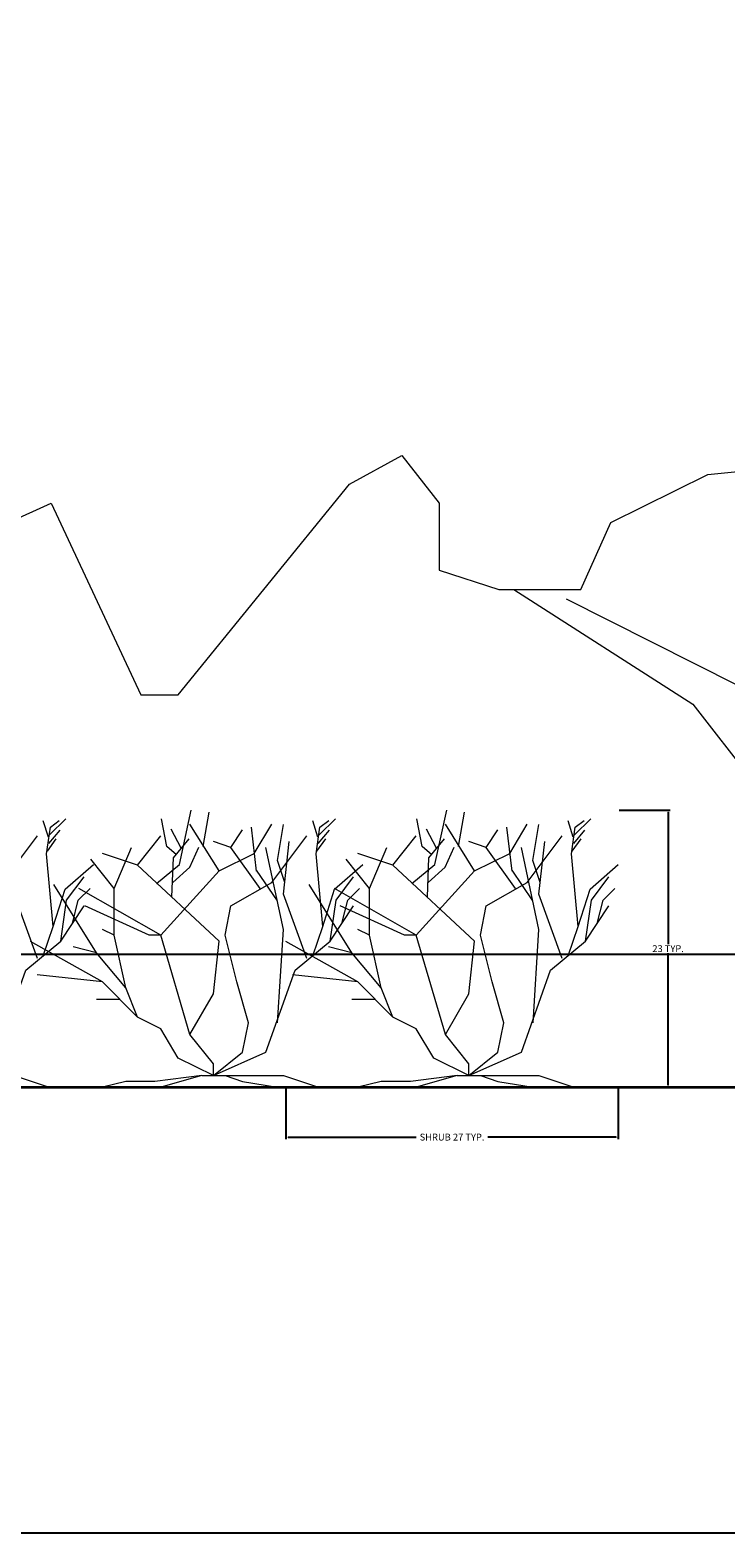
# Model space of a CAD drawing. Units: inches. Extents: x -26 to 776, y -22 to 650.
# Tile 45 of 62: x 584 to 642, y -22 to 102. Entities that reach past the tile are written whole.
import ezdxf

# ---------------------------------------------------------------- set-up
doc = ezdxf.new("R2010")
doc.units = ezdxf.units.IN
doc.header["$MEASUREMENT"] = 0
for name, color, linetype, lineweight in [('A-ANNO-DIMS', 2, 'Continuous', 18), ('C-TOPO', 7, 'Continuous', 35), ('L-PLNT-SHRB', 94, 'Continuous', 13), ('L-PLNT-TREE', 94, 'Continuous', 18)]:
    doc.layers.add(name, color=color, linetype=linetype, lineweight=lineweight)
doc.styles.get("Standard").update_dxf_attribs({"font": 'arial.ttf'})
doc.dimstyles.get("Standard").update_dxf_attribs({"dimtxt": 0.5625, "dimasz": 0.18, "dimexe": 0.18, "dimexo": 0.0625, "dimgap": 0.09, "dimtad": 0, "dimtih": 1, "dimtoh": 1, "dimdec": 4, "dimzin": 0, "dimdsep": 46, "dimlunit": 4, "dimtxsty": 'Standard', "dimcen": 0.09, "dimadec": 0, "dimazin": 0, "dimtfac": 1, "dimtdec": 4, "dimtofl": 0, "dimtmove": 0, "dimatfit": 3, "dimfxl": 1, "dimtolj": 1, "dimtzin": 0, "dimarcsym": 0})

# ---------------------------------------------------------------- blocks, each defined once
blk = doc.blocks.new('Tree - type 3 evergreen elevation')
for points in [[(-41.4085, 64.6985), (-44.3346, 59.8898), (-42.2089, 60.1377), (-42.5159, 55.7849), (-49.6039, 46.4502), (-58.2307, 45.8972), (-62.1127, 43.6853), (-68.5828, 36.4966), (-65.9947, 32.0727), (-50.0352, 32.6257), (-47.0159, 30.4138), (-39.6831, 33.7317), (-34.507, 22.6721), (-32.3504, 22.6721), (-22.4296, 34.8376), (-19.4102, 36.4966), (-17.2536, 33.7317), (-17.2536, 29.8608), (-13.8028, 28.7549), (-9.0581, 28.7549), (-7.3328, 32.6257), (-1.7254, 35.3906), (3.8821, 35.9436)], [(-9.9208, 28.2019), (0, 23.2251), (3.4507, 19.9072), (4.7447, 15.4834), (8.6267, 27.0959), (6.4701, 37.6025)], [(-12.9401, 28.7549), (-2.588, 22.1191), (0.8626, 17.6953), (1.7253, 11.6125), (0, 0)]]:
    blk.add_lwpolyline(points)
blk = doc.blocks.new('Shrub - elevation')
for p, q in [((-11.433, 18.289), (-10.457, 22.749)), ((-9.48, 19.775), (-8.992, 22.592)), ((-12.471, 19.775), (-12.898, 22.044)), ((-11.28, 19.619), (-12.104, 21.184)), ((-8.16, 17.76), (-10.56, 21.6)), ((-7.2, 19.68), (-6.24, 21.12)), ((-5.086, 17.741), (-5.513, 21.34)), ((-5.28, 19.2), (-3.84, 21.6)), ((-3.377, 18.602), (-2.888, 21.575)), ((-0.508, 21.888), (-0.081, 20.558)), ((-0.203, 19.149), (0.102, 21.34)), ((-0.02, 20.01), (0.896, 21.105)), ((0.041, 20.714), (1.384, 22.044)), ((0.102, 21.34), (0.835, 21.888)), ((-14.88, 18.24), (-12.96, 20.64)), ((-11.921, 18.836), (-10.64, 20.401)), ((-7.2, 19.68), (-8.64, 20.16)), ((-3.84, 16.8), (-0.96, 20.64)), ((-2.88, 15.84), (-2.4, 20.16)), ((-0.142, 19.384), (0.59, 20.401)), ((-16.8, 16.32), (-18.72, 18.72)), ((-14.88, 18.24), (-17.76, 19.2)), ((-16.8, 16.32), (-15.36, 19.68)), ((-11.677, 19.071), (-12.471, 19.775)), ((-12.043, 15.628), (-11.921, 18.836)), ((-10.579, 18.054), (-9.846, 19.697)), ((-8.16, 17.76), (-5.28, 19.2)), ((-4.8, 16.32), (-7.2, 19.68)), ((-2.88, 12.96), (-4.32, 19.68)), ((-2.766, 16.802), (-3.377, 18.602)), ((0.346, 13.203), (-0.203, 19.149)), ((-8.16, 12), (-14.88, 18.24)), ((-13.325, 16.724), (-11.433, 18.289)), ((-12.96, 12.48), (-8.16, 17.76)), ((-11.982, 16.802), (-10.579, 18.054)), ((-3.377, 15.315), (-5.086, 17.819)), ((1.323, 16.254), (3.642, 18.289)), ((-18.24, 11.04), (-21.755, 16.655)), ((-12.96, 12.48), (-19.68, 16.32)), ((-16.8, 12.48), (-16.8, 16.32)), ((-7.2, 14.88), (-3.84, 16.8)), ((0.346, 13.203), (1.323, 16.254)), ((1.44, 15.36), (2.88, 17.28)), ((2.4, 15.36), (3.36, 16.32)), ((-13.92, 12.48), (-19.2, 14.88)), ((-7.68, 12.48), (-7.2, 14.88)), ((-0.96, 10.56), (-2.88, 15.84)), ((0.96, 12), (1.44, 15.36)), ((0.96, 12), (2.88, 14.88)), ((1.92, 13.44), (2.4, 15.36)), ((-16.8, 12.48), (-17.76, 12.96)), ((-15.84, 8.16), (-16.8, 12.48)), ((-12.96, 12.48), (-13.92, 12.48)), ((-10.56, 4.32), (-12.96, 12.48)), ((-6.72, 8.64), (-7.68, 12.48)), ((-3.36, 5.28), (-2.88, 12.96)), ((-0.48, 10.8), (0.346, 13.203)), ((-17.76, 8.64), (-23.663, 11.961)), ((-18.24, 11.04), (-20.16, 11.52)), ((-8.64, 7.68), (-8.16, 12)), ((-1.92, 9.6), (0.96, 12)), ((-15.84, 8.16), (-18.24, 11.04)), ((-17.76, 8.64), (-23.128, 9.222)), ((-4.32, 2.88), (-1.92, 9.6)), ((-14.88, 5.76), (-17.76, 8.64)), ((-14.88, 5.76), (-15.84, 8.16)), ((-10.56, 4.32), (-8.64, 7.68)), ((-5.76, 5.28), (-6.72, 8.64)), ((-16.32, 7.2), (-18.24, 7.2)), ((-12.96, 4.8), (-14.88, 5.76)), ((-6.24, 2.88), (-5.76, 5.28)), ((-11.52, 2.4), (-12.96, 4.8)), ((-8.64, 1.92), (-10.56, 4.32)), ((-8.64, 0.96), (-4.32, 2.88)), ((-8.64, 0.96), (-6.24, 2.88)), ((-8.64, 0.96), (-11.52, 2.4)), ((-8.64, 0.96), (-8.64, 1.92)), ((-15.84, 0.48), (-17.76, 0)), ((-13.44, 0.48), (-15.84, 0.48)), ((-9.6, 0.96), (-13.44, 0.48)), ((-9.6, 0.96), (-12.96, 0)), ((-9.6, 0.96), (-7.68, 0.96)), ((-8.64, 0.96), (-2.88, 0.96)), ((-7.68, 0.96), (-6.24, 0.48)), ((-6.24, 0.48), (-3.36, 0)), ((-2.88, 0.96), (0, 0))]:
    blk.add_line(p, q)
blk = doc.blocks.new('*D11')
at = {"layer": 'A-ANNO-DIMS', "color": 0, "lineweight": -2, "transparency": 16777216}
for p, q in [((605.39, 15.42), (605.39, 11.21)), ((632.7, 15.42), (632.7, 11.21)), ((605.57, 11.39), (616.1, 11.39)), ((632.52, 11.39), (621.99, 11.39))]:
    blk.add_line(p, q, dxfattribs=at)
at = {"layer": 'A-ANNO-DIMS', "color": 0, "transparency": 16777216}
for points in [[(605.57, 11.42), (605.57, 11.36), (605.39, 11.39)], [(632.52, 11.42), (632.52, 11.36), (632.7, 11.39)]]:
    blk.add_solid(points, dxfattribs=at)
at = {"layer": 'Defpoints', "color": 0, "transparency": 16777216}
for p in [(605.39, 15.48), (632.7, 15.48), (632.7, 11.39)]:
    blk.add_point(p, dxfattribs=at)
at = {"layer": 'A-ANNO-DIMS', "color": 0, "transparency": 16777216, "insert": (619.04, 11.39), "char_height": 0.5625, "attachment_point": 5}
blk.add_mtext('\\A1;SHRUB 27 TYP.', dxfattribs=at)
blk = doc.blocks.new('*D12')
at = {"layer": 'A-ANNO-DIMS', "color": 0, "lineweight": -2, "transparency": 16777216}
for p, q in [((632.76, 38.23), (636.97, 38.23)), ((636.79, 38.05), (636.79, 27.23)), ((636.79, 15.66), (636.79, 26.48)), ((632.76, 15.48), (636.97, 15.48))]:
    blk.add_line(p, q, dxfattribs=at)
at = {"layer": 'A-ANNO-DIMS', "color": 0, "transparency": 16777216}
for points in [[(636.76, 38.05), (636.82, 38.05), (636.79, 38.23)], [(636.76, 15.66), (636.82, 15.66), (636.79, 15.48)]]:
    blk.add_solid(points, dxfattribs=at)
at = {"layer": 'Defpoints', "color": 0, "transparency": 16777216}
for p in [(632.7, 38.23), (636.79, 38.23), (632.7, 15.48)]:
    blk.add_point(p, dxfattribs=at)
at = {"layer": 'A-ANNO-DIMS', "color": 0, "transparency": 16777216, "insert": (636.79, 26.86), "char_height": 0.5625, "attachment_point": 5}
blk.add_mtext('\\A1;23 TYP.', dxfattribs=at)
blk = doc.blocks.new('*D13')
at = {"layer": 'A-ANNO-DIMS', "color": 0, "lineweight": -2, "transparency": 16777216}
for p, q in [((738.75, 50.79), (738.75, -21.31)), ((11.11, 15.42), (11.11, -21.31)), ((11.29, -21.13), (373.89, -21.13)), ((738.57, -21.13), (375.97, -21.13))]:
    blk.add_line(p, q, dxfattribs=at)
at = {"layer": 'A-ANNO-DIMS', "color": 0, "transparency": 16777216}
for points in [[(11.29, -21.1), (11.29, -21.16), (11.11, -21.13)], [(738.57, -21.1), (738.57, -21.16), (738.75, -21.13)]]:
    blk.add_solid(points, dxfattribs=at)
at = {"layer": 'Defpoints', "color": 0, "transparency": 16777216}
for p in [(738.75, 50.85), (11.11, 15.48), (738.75, -21.13)]:
    blk.add_point(p, dxfattribs=at)
at = {"layer": 'A-ANNO-DIMS', "color": 0, "transparency": 16777216, "insert": (374.93, -21.13), "char_height": 0.562, "attachment_point": 5}
blk.add_mtext('\\A1;727.6', dxfattribs=at)
blk = doc.blocks.new('*D20')
at = {"layer": 'A-ANNO-DIMS', "color": 0, "lineweight": -2, "transparency": 16777216}
for p, q in [((425.81, 455.47), (775.34, 455.47)), ((775.16, 455.29), (775.16, 235.85)), ((775.16, 15.66), (775.16, 235.1)), ((425.81, 15.48), (775.34, 15.48))]:
    blk.add_line(p, q, dxfattribs=at)
at = {"layer": 'A-ANNO-DIMS', "color": 0, "transparency": 16777216}
for points in [[(775.13, 455.29), (775.19, 455.29), (775.16, 455.47)], [(775.13, 15.66), (775.19, 15.66), (775.16, 15.48)]]:
    blk.add_solid(points, dxfattribs=at)
at = {"layer": 'Defpoints', "color": 0, "transparency": 16777216}
for p in [(425.74, 455.47), (775.16, 455.47), (425.74, 15.48)]:
    blk.add_point(p, dxfattribs=at)
at = {"layer": 'A-ANNO-DIMS', "color": 0, "transparency": 16777216, "insert": (775.16, 235.48), "char_height": 0.562, "attachment_point": 5}
blk.add_mtext('\\A1;440', dxfattribs=at)
blk = doc.blocks.new('*D30')
at = {"layer": 'A-ANNO-DIMS', "color": 0, "lineweight": -2, "transparency": 16777216}
for p, q in [((280.68, 144.84), (775.34, 144.84)), ((775.16, 144.66), (775.16, 86.01)), ((775.16, 26.6), (775.16, 85.25)), ((280.68, 26.42), (775.34, 26.42))]:
    blk.add_line(p, q, dxfattribs=at)
at = {"layer": 'A-ANNO-DIMS', "color": 0, "transparency": 16777216}
for points in [[(775.13, 144.66), (775.19, 144.66), (775.16, 144.84)], [(775.13, 26.6), (775.19, 26.6), (775.16, 26.42)]]:
    blk.add_solid(points, dxfattribs=at)
at = {"layer": 'Defpoints', "color": 0, "transparency": 16777216}
for p in [(280.62, 144.84), (775.16, 144.84), (280.62, 26.42)]:
    blk.add_point(p, dxfattribs=at)
at = {"layer": 'A-ANNO-DIMS', "color": 0, "transparency": 16777216, "insert": (775.16, 85.63), "char_height": 0.562, "attachment_point": 5}
blk.add_mtext('\\A1;118.41', dxfattribs=at)
blk = doc.blocks.new('*D38')
at = {"layer": 'A-ANNO-DIMS', "color": 0, "lineweight": -2, "transparency": 16777216}
for p, q in [((280.68, 26.42), (775.34, 26.42)), ((775.16, 26.24), (775.16, 21.33)), ((775.16, 15.66), (775.16, 20.58)), ((289.3, 15.48), (775.34, 15.48))]:
    blk.add_line(p, q, dxfattribs=at)
at = {"layer": 'A-ANNO-DIMS', "color": 0, "transparency": 16777216}
for points in [[(775.13, 26.24), (775.19, 26.24), (775.16, 26.42)], [(775.13, 15.66), (775.19, 15.66), (775.16, 15.48)]]:
    blk.add_solid(points, dxfattribs=at)
at = {"layer": 'Defpoints', "color": 0, "transparency": 16777216}
for p in [(280.62, 26.42), (775.16, 26.42), (289.24, 15.48)]:
    blk.add_point(p, dxfattribs=at)
at = {"layer": 'A-ANNO-DIMS', "color": 0, "transparency": 16777216, "insert": (775.16, 20.95), "char_height": 0.562, "attachment_point": 5}
blk.add_mtext('\\A1;10.942', dxfattribs=at)
blk = doc.blocks.new('*D45')
at = {"layer": 'A-ANNO-DIMS', "color": 0, "lineweight": -2, "transparency": 16777216}
for p, q in [((507.74, 408.64), (775.34, 408.64)), ((775.16, 408.46), (775.16, 212.44)), ((775.16, 15.66), (775.16, 211.68)), ((586, 15.48), (775.34, 15.48))]:
    blk.add_line(p, q, dxfattribs=at)
at = {"layer": 'A-ANNO-DIMS', "color": 0, "transparency": 16777216}
for points in [[(775.13, 408.46), (775.19, 408.46), (775.16, 408.64)], [(775.13, 15.66), (775.19, 15.66), (775.16, 15.48)]]:
    blk.add_solid(points, dxfattribs=at)
at = {"layer": 'Defpoints', "color": 0, "transparency": 16777216}
for p in [(507.68, 408.64), (775.16, 408.64), (585.94, 15.48)]:
    blk.add_point(p, dxfattribs=at)
at = {"layer": 'A-ANNO-DIMS', "color": 0, "transparency": 16777216, "insert": (775.16, 212.06), "char_height": 0.562, "attachment_point": 5}
blk.add_mtext('\\A1;393.16', dxfattribs=at)
blk = doc.blocks.new('*D48')
at = {"layer": 'A-ANNO-DIMS', "color": 0, "lineweight": -2, "transparency": 16777216}
for p, q in [((545.03, 67.41), (545.03, 649.86)), ((738.75, 50.91), (738.75, 649.86)), ((545.21, 649.68), (640.88, 649.68)), ((738.57, 649.68), (642.9, 649.68))]:
    blk.add_line(p, q, dxfattribs=at)
at = {"layer": 'A-ANNO-DIMS', "color": 0, "transparency": 16777216}
for points in [[(545.21, 649.71), (545.21, 649.65), (545.03, 649.68)], [(738.57, 649.71), (738.57, 649.65), (738.75, 649.68)]]:
    blk.add_solid(points, dxfattribs=at)
at = {"layer": 'Defpoints', "color": 0, "transparency": 16777216}
for p in [(738.75, 649.68), (545.03, 67.35), (738.75, 50.85)]:
    blk.add_point(p, dxfattribs=at)
at = {"layer": 'A-ANNO-DIMS', "color": 0, "transparency": 16777216, "insert": (641.89, 649.68), "char_height": 0.562, "attachment_point": 5}
blk.add_mtext('\\A1;193.7', dxfattribs=at)

msp = doc.modelspace()

# ---------------------------------------------------------------- linework, layer by layer
at = {"layer": 'C-TOPO'}
msp.add_line((425.7434, 15.4824), (677.9037, 15.4824), dxfattribs=at)

# ---------------------------------------------------------------- block references
at = {"layer": 'L-PLNT-SHRB'}
for p in [(585.9354, 15.4824), (608.0702, 15.4824), (629.0552, 15.4824)]:
    msp.add_blockref('Shrub - elevation', p, dxfattribs=at)
at = {"layer": 'L-PLNT-TREE', "xscale": 1.421226385586178, "yscale": 1.421226385586178, "zscale": 1.421226385586178}
msp.add_blockref('Tree - type 3 evergreen elevation', (642.5048, 15.4824), dxfattribs=at)

# ---------------------------------------------------------------- dimensions: what is measured, and where the dimension line sits
at = {"layer": 'A-ANNO-DIMS'}
for base, p1, picture, middle in [((738.7503, 649.6763), (545.0331, 67.3523), '*D48', (641.8917, 649.6763)), ((738.7503, -21.1349), (11.1074, 15.4824), '*D13', (374.9289, -21.1349))]:
    dim = msp.add_linear_dim(base=base, p1=p1, p2=(738.7503, 50.8482), dimstyle='Standard', override={"dimdec": 1, "dimlfac": 1, "dimrnd": 0, "dimzin": 0, "dimdsep": 46, "dimlunit": 2}, dxfattribs=at)
    dim.commit()
    dim.dimension.update_dxf_attribs({"geometry": picture, "text_midpoint": middle})
for base, p1, p2, override, picture, middle in [((775.1553, 455.4717), (425.7434, 15.4824), (425.7434, 455.4717), {"dimdec": 0, "dimlfac": 1, "dimrnd": 0, "dimzin": 0, "dimdsep": 46, "dimlunit": 2}, '*D20', (775.1553, 235.477)), ((775.1553, 408.6389), (585.9354, 15.4824), (507.6759, 408.6389), {"dimdec": 2, "dimlfac": 1, "dimrnd": 0, "dimzin": 0, "dimdsep": 46, "dimlunit": 2}, '*D45', (775.1553, 212.0606)), ((775.1553, 144.8359), (280.6173, 26.4239), (280.6173, 144.8359), {"dimdec": 2, "dimlfac": 1, "dimrnd": 0, "dimzin": 0, "dimdsep": 46, "dimlunit": 2}, '*D30', (775.1553, 85.6299)), ((775.15535, 26.4239), (289.24236, 15.48237), (280.61732, 26.4239), {"dimdec": 3, "dimlfac": 1, "dimrnd": 0, "dimzin": 0, "dimdsep": 46, "dimlunit": 2}, '*D38', (775.15535, 20.95313))]:
    dim = msp.add_linear_dim(base=base, p1=p1, p2=p2, angle=90, dimstyle='Standard', override=override, dxfattribs=at)
    dim.commit()
    dim.dimension.update_dxf_attribs({"geometry": picture, "text_midpoint": middle})
dim = msp.add_linear_dim(base=(636.7929, 38.2314), p1=(632.6972, 15.4824), p2=(632.6972, 38.2314), angle=90, text='<> TYP.', dimstyle='Standard', override={"dimdec": 0, "dimlfac": 1, "dimrnd": 0, "dimzin": 0, "dimdsep": 46, "dimlunit": 2}, dxfattribs=at)
dim.commit()
dim.dimension.update_dxf_attribs({"geometry": '*D12', "text_midpoint": (636.7929, 26.8569)})
dim = msp.add_linear_dim(base=(632.6972, 11.3866), p1=(605.3922, 15.4824), p2=(632.6972, 15.4824), text='SHRUB <> TYP.', dimstyle='Standard', override={"dimdec": 0, "dimlfac": 1, "dimrnd": 0, "dimzin": 0, "dimdsep": 46, "dimlunit": 2}, dxfattribs=at)
dim.commit()
dim.dimension.update_dxf_attribs({"geometry": '*D11', "text_midpoint": (619.0447, 11.3866)})

doc.saveas('drawing.dxf')
